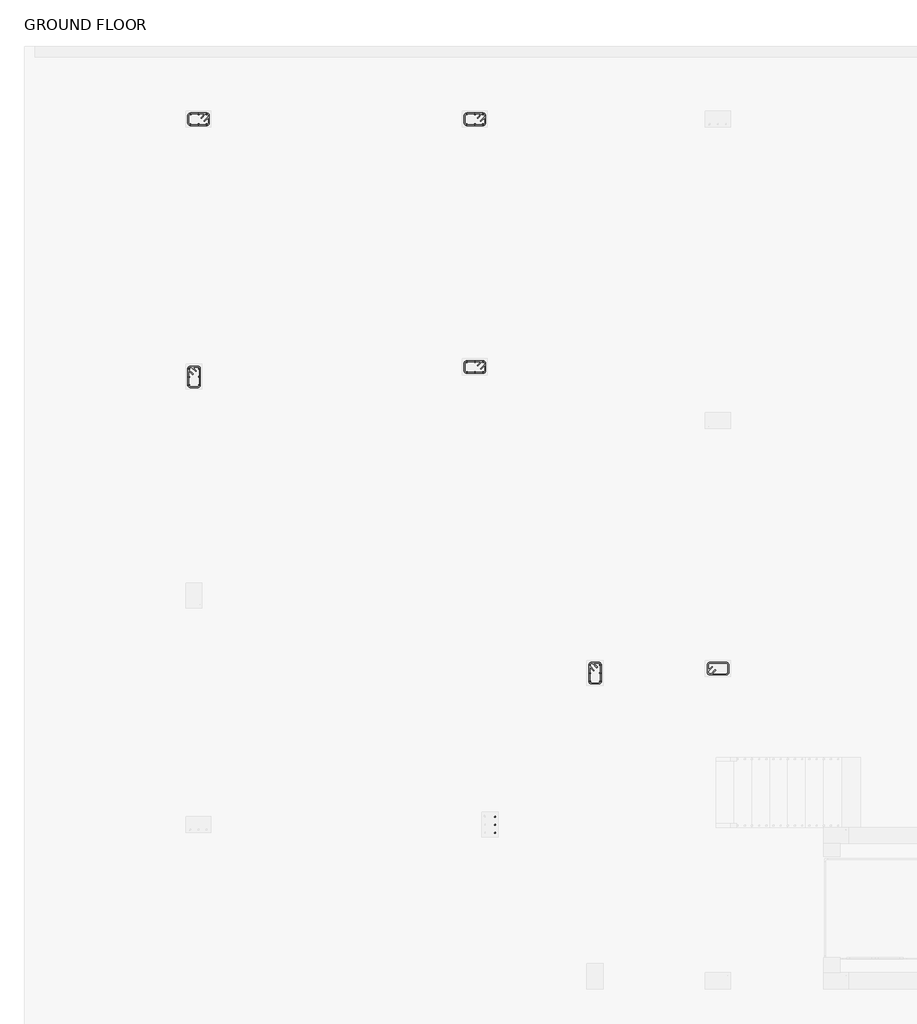
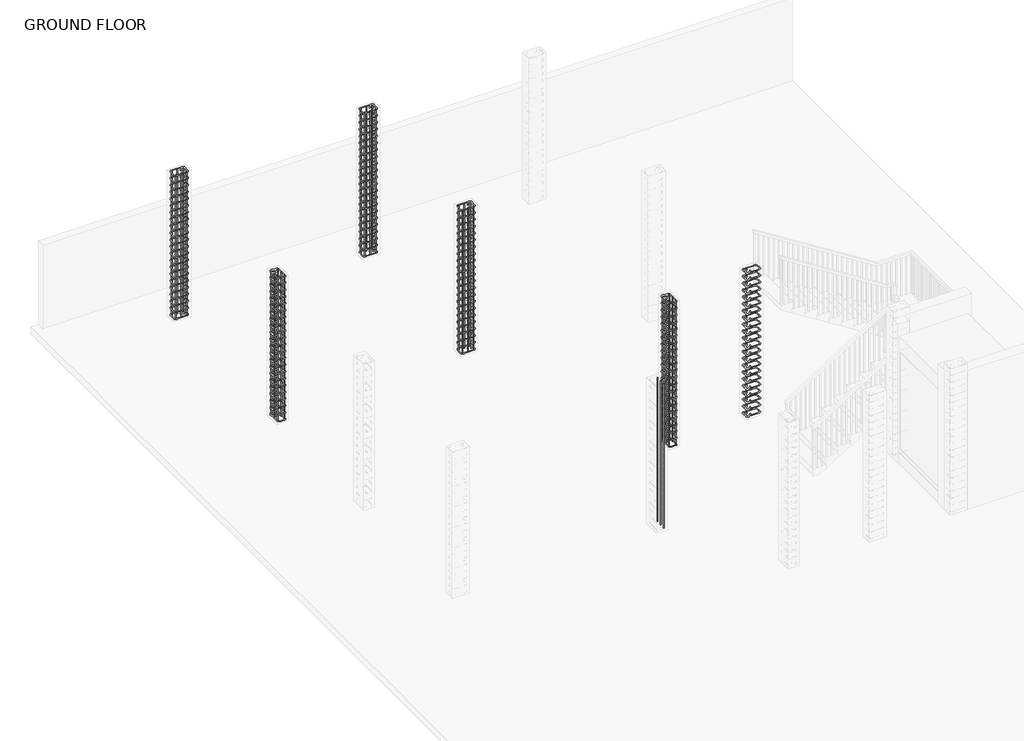
# One storey, part 6 of 7: 17 reinforcing bars.
"""IFC4 building model written with IfcOpenShell, lengths in millimetres."""

from ifc_helpers import new_model, si_unit, point, frame, origin, place, context, project, spatial, polyline, circle_curve, trimmed, segment, composite_curve, source, transform, mapped, element, save
from ifc_brep_helpers import swept_disk

model = new_model("IFC4")

# Units and contexts
model_context = context("Model", 3, world=origin())
ifc_project = project(units=[si_unit("LENGTHUNIT", "METRE", prefix="MILLI")], contexts=[model_context])

# Site, building, storey
site = spatial("IfcSite", under=ifc_project)
building = spatial("IfcBuilding", under=site)
storey = spatial("IfcBuildingStorey", under=building, Name="GROUND FLOOR", Elevation=0.0)

# Reinforcing bars
placement = place(None, origin())
reinforcing_bar_shape = source(origin(), model_context, "Body", "SolidModel", [
    swept_disk(composite_curve([segment(polyline([(-6036.4155558, 10049.1290376, 3168.65), (-5982.534019, 10103.0105743, 3168.65)]), True, "CONTINUOUS"), segment(trimmed(circle_curve(frame((-5960.0833787, 10080.559934, 3168.65), z_axis=(0.0, 0.0, -1.0), x_axis=(-22.450640299999577, 22.450640299999577, 0.0)), 31.75), [point((-5982.534019, 10103.0105743, 3168.65))], [point((-5928.3333787, 10080.559934, 3168.65))], True, "CARTESIAN"), True, "CONTINUOUS"), segment(polyline([(-5928.3333787, 10080.559934, 3168.65), (-5928.3333787, 9978.959934, 3168.65)]), True, "CONTINUOUS"), segment(trimmed(circle_curve(frame((-5960.0833787, 9978.959934, 3168.65), z_axis=(0.0, 0.0, -1.0), x_axis=(31.75, 0.0, 0.0)), 31.75), [point((-5928.3333787, 9978.959934, 3168.65))], [point((-5960.0833787, 9947.209934, 3168.65))], True, "CARTESIAN"), True, "CONTINUOUS"), segment(polyline([(-5960.0833787, 9947.209934, 3168.65), (-6188.6833787, 9947.209934, 3168.65)]), True, "CONTINUOUS"), segment(trimmed(circle_curve(frame((-6188.6833787, 9978.8664139, 3171.0851138), z_axis=(0.0, 0.07669649888473773, -0.9970544855015816), x_axis=(0.0, -31.656479899998885, -2.4351137999997263)), 31.75), [point((-6188.6833787, 9947.209934, 3168.65))], [point((-6220.4333787, 9978.8664139, 3171.0851138))], True, "CARTESIAN"), True, "CONTINUOUS"), segment(polyline([(-6220.4333787, 9978.8664139, 3171.0851138), (-6220.4333787, 10080.6534541, 3178.9148862)]), True, "CONTINUOUS"), segment(trimmed(circle_curve(frame((-6188.6833787, 10080.6534541, 3178.9148862), z_axis=(0.0, 0.07669649888473773, -0.9970544855015816), x_axis=(-31.75, 0.0, 0.0)), 31.75), [point((-6220.4333787, 10080.6534541, 3178.9148862))], [point((-6188.6833787, 10112.309934, 3181.35))], True, "CARTESIAN"), True, "CONTINUOUS"), segment(polyline([(-6188.6833787, 10112.309934, 3181.35), (-5960.0833787, 10112.309934, 3181.35)]), True, "CONTINUOUS"), segment(trimmed(circle_curve(frame((-5960.0833787, 10080.559934, 3181.35), z_axis=(0.0, 0.0, -1.0), x_axis=(0.0, 31.75, 0.0)), 31.75), [point((-5960.0833787, 10112.309934, 3181.35))], [point((-5937.6327384, 10058.1092937, 3181.35))], True, "CARTESIAN"), True, "CONTINUOUS"), segment(polyline([(-5937.6327384, 10058.1092937, 3181.35), (-5991.5142752, 10004.227757, 3181.35)]), True, "CONTINUOUS")], self_intersect=False), 6.35),
])
element("IfcReinforcingBar", 1, at=placement, inside=storey, context=model_context, shape_type="MappedRepresentation", body=[
    mapped(reinforcing_bar_shape, transform((0.0, 0.0, 0.0), x_axis=(1.0, 0.0, 0.0), y_axis=(0.0, 1.0, 0.0), z_axis=(0.0, 0.0, 1.0))),
    mapped(reinforcing_bar_shape, transform((0.0, 0.0, -149.3761905), x_axis=(1.0, 0.0, 0.0), y_axis=(0.0, 1.0, 0.0), z_axis=(0.0, 0.0, 1.0))),
    mapped(reinforcing_bar_shape, transform((0.0, 0.0, -298.752381), x_axis=(1.0, 0.0, 0.0), y_axis=(0.0, 1.0, 0.0), z_axis=(0.0, 0.0, 1.0))),
    mapped(reinforcing_bar_shape, transform((0.0, 0.0, -448.1285714), x_axis=(1.0, 0.0, 0.0), y_axis=(0.0, 1.0, 0.0), z_axis=(0.0, 0.0, 1.0))),
    mapped(reinforcing_bar_shape, transform((0.0, 0.0, -597.5047619), x_axis=(1.0, 0.0, 0.0), y_axis=(0.0, 1.0, 0.0), z_axis=(0.0, 0.0, 1.0))),
    mapped(reinforcing_bar_shape, transform((0.0, 0.0, -746.8809524), x_axis=(1.0, 0.0, 0.0), y_axis=(0.0, 1.0, 0.0), z_axis=(0.0, 0.0, 1.0))),
    mapped(reinforcing_bar_shape, transform((0.0, 0.0, -896.2571429), x_axis=(1.0, 0.0, 0.0), y_axis=(0.0, 1.0, 0.0), z_axis=(0.0, 0.0, 1.0))),
    mapped(reinforcing_bar_shape, transform((0.0, 0.0, -1045.6333333), x_axis=(1.0, 0.0, 0.0), y_axis=(0.0, 1.0, 0.0), z_axis=(0.0, 0.0, 1.0))),
    mapped(reinforcing_bar_shape, transform((0.0, 0.0, -1195.0095238), x_axis=(1.0, 0.0, 0.0), y_axis=(0.0, 1.0, 0.0), z_axis=(0.0, 0.0, 1.0))),
    mapped(reinforcing_bar_shape, transform((0.0, 0.0, -1344.3857143), x_axis=(1.0, 0.0, 0.0), y_axis=(0.0, 1.0, 0.0), z_axis=(0.0, 0.0, 1.0))),
    mapped(reinforcing_bar_shape, transform((0.0, 0.0, -1493.7619048), x_axis=(1.0, 0.0, 0.0), y_axis=(0.0, 1.0, 0.0), z_axis=(0.0, 0.0, 1.0))),
    mapped(reinforcing_bar_shape, transform((0.0, 0.0, -1643.1380952), x_axis=(1.0, 0.0, 0.0), y_axis=(0.0, 1.0, 0.0), z_axis=(0.0, 0.0, 1.0))),
    mapped(reinforcing_bar_shape, transform((0.0, 0.0, -1792.5142857), x_axis=(1.0, 0.0, 0.0), y_axis=(0.0, 1.0, 0.0), z_axis=(0.0, 0.0, 1.0))),
    mapped(reinforcing_bar_shape, transform((0.0, 0.0, -1941.8904762), x_axis=(1.0, 0.0, 0.0), y_axis=(0.0, 1.0, 0.0), z_axis=(0.0, 0.0, 1.0))),
    mapped(reinforcing_bar_shape, transform((0.0, 0.0, -2091.2666667), x_axis=(1.0, 0.0, 0.0), y_axis=(0.0, 1.0, 0.0), z_axis=(0.0, 0.0, 1.0))),
    mapped(reinforcing_bar_shape, transform((0.0, 0.0, -2240.6428571), x_axis=(1.0, 0.0, 0.0), y_axis=(0.0, 1.0, 0.0), z_axis=(0.0, 0.0, 1.0))),
    mapped(reinforcing_bar_shape, transform((0.0, 0.0, -2390.0190476), x_axis=(1.0, 0.0, 0.0), y_axis=(0.0, 1.0, 0.0), z_axis=(0.0, 0.0, 1.0))),
    mapped(reinforcing_bar_shape, transform((0.0, 0.0, -2539.3952381), x_axis=(1.0, 0.0, 0.0), y_axis=(0.0, 1.0, 0.0), z_axis=(0.0, 0.0, 1.0))),
    mapped(reinforcing_bar_shape, transform((0.0, 0.0, -2688.7714286), x_axis=(1.0, 0.0, 0.0), y_axis=(0.0, 1.0, 0.0), z_axis=(0.0, 0.0, 1.0))),
    mapped(reinforcing_bar_shape, transform((0.0, 0.0, -2838.147619), x_axis=(1.0, 0.0, 0.0), y_axis=(0.0, 1.0, 0.0), z_axis=(0.0, 0.0, 1.0))),
    mapped(reinforcing_bar_shape, transform((0.0, 0.0, -2987.5238095), x_axis=(1.0, 0.0, 0.0), y_axis=(0.0, 1.0, 0.0), z_axis=(0.0, 0.0, 1.0))),
    mapped(reinforcing_bar_shape, transform((0.0, 0.0, -3136.9), x_axis=(1.0, 0.0, 0.0), y_axis=(0.0, 1.0, 0.0), z_axis=(0.0, 0.0, 1.0))),
])
reinforcing_bar_2_shape = source(origin(), model_context, "Body", "SolidModel", [
    swept_disk(composite_curve([segment(polyline([(-5960.0833787, 9959.909934, 3175.0), (-5960.0833787, 9959.909934, 25.4)]), True, "CONTINUOUS")], self_intersect=False), 6.35),
])
element("IfcReinforcingBar", 2, at=placement, inside=storey, context=model_context, shape_type="MappedRepresentation", body=[
    mapped(reinforcing_bar_2_shape, transform((0.0, 0.0, 0.0), x_axis=(1.0, 0.0, 0.0), y_axis=(0.0, 1.0, 0.0), z_axis=(0.0, 0.0, 1.0))),
    mapped(reinforcing_bar_2_shape, transform((-114.3, 0.0, 0.0), x_axis=(1.0, 0.0, 0.0), y_axis=(0.0, 1.0, 0.0), z_axis=(0.0, 0.0, 1.0))),
    mapped(reinforcing_bar_2_shape, transform((-228.6, 0.0, 0.0), x_axis=(1.0, 0.0, 0.0), y_axis=(0.0, 1.0, 0.0), z_axis=(0.0, 0.0, 1.0))),
])
reinforcing_bar_3_shape = source(origin(), model_context, "Body", "SolidModel", [
    swept_disk(composite_curve([segment(polyline([(-5960.0833787, 10099.609934, 25.4), (-5960.0833787, 10099.609934, 3175.0)]), True, "CONTINUOUS")], self_intersect=False), 6.35),
])
element("IfcReinforcingBar", 3, at=placement, inside=storey, context=model_context, shape_type="MappedRepresentation", body=[
    mapped(reinforcing_bar_3_shape, transform((0.0, 0.0, 0.0), x_axis=(1.0, 0.0, 0.0), y_axis=(0.0, 1.0, 0.0), z_axis=(0.0, 0.0, 1.0))),
    mapped(reinforcing_bar_3_shape, transform((-114.3, 0.0, 0.0), x_axis=(1.0, 0.0, 0.0), y_axis=(0.0, 1.0, 0.0), z_axis=(0.0, 0.0, 1.0))),
    mapped(reinforcing_bar_3_shape, transform((-228.6, 0.0, 0.0), x_axis=(1.0, 0.0, 0.0), y_axis=(0.0, 1.0, 0.0), z_axis=(0.0, 0.0, 1.0))),
])
reinforcing_bar_4_shape = source(origin(), model_context, "Body", "SolidModel", [
    swept_disk(composite_curve([segment(polyline([(-2124.8155558, 10049.1290376, 3168.65), (-2070.934019, 10103.0105743, 3168.65)]), True, "CONTINUOUS"), segment(trimmed(circle_curve(frame((-2048.4833787, 10080.559934, 3168.65), z_axis=(0.0, 0.0, -1.0), x_axis=(-22.450640300000032, 22.450640299999577, 0.0)), 31.75), [point((-2070.934019, 10103.0105743, 3168.65))], [point((-2016.7333787, 10080.559934, 3168.65))], True, "CARTESIAN"), True, "CONTINUOUS"), segment(polyline([(-2016.7333787, 10080.559934, 3168.65), (-2016.7333787, 9978.959934, 3168.65)]), True, "CONTINUOUS"), segment(trimmed(circle_curve(frame((-2048.4833787, 9978.959934, 3168.65), z_axis=(0.0, 0.0, -1.0), x_axis=(31.749999999999773, 0.0, 0.0)), 31.75), [point((-2016.7333787, 9978.959934, 3168.65))], [point((-2048.4833787, 9947.209934, 3168.65))], True, "CARTESIAN"), True, "CONTINUOUS"), segment(polyline([(-2048.4833787, 9947.209934, 3168.65), (-2277.0833787, 9947.209934, 3168.65)]), True, "CONTINUOUS"), segment(trimmed(circle_curve(frame((-2277.0833787, 9978.8664139, 3171.0851138), z_axis=(0.0, 0.07669649888473773, -0.9970544855015816), x_axis=(0.0, -31.656479899998885, -2.4351137999997263)), 31.75), [point((-2277.0833787, 9947.209934, 3168.65))], [point((-2308.8333787, 9978.8664139, 3171.0851138))], True, "CARTESIAN"), True, "CONTINUOUS"), segment(polyline([(-2308.8333787, 9978.8664139, 3171.0851138), (-2308.8333787, 10080.6534541, 3178.9148862)]), True, "CONTINUOUS"), segment(trimmed(circle_curve(frame((-2277.0833787, 10080.6534541, 3178.9148862), z_axis=(0.0, 0.07669649888473773, -0.9970544855015816), x_axis=(-31.75, 0.0, 0.0)), 31.75), [point((-2308.8333787, 10080.6534541, 3178.9148862))], [point((-2277.0833787, 10112.309934, 3181.35))], True, "CARTESIAN"), True, "CONTINUOUS"), segment(polyline([(-2277.0833787, 10112.309934, 3181.35), (-2048.4833787, 10112.309934, 3181.35)]), True, "CONTINUOUS"), segment(trimmed(circle_curve(frame((-2048.4833787, 10080.559934, 3181.35), z_axis=(0.0, 0.0, -1.0), x_axis=(0.0, 31.75, 0.0)), 31.75), [point((-2048.4833787, 10112.309934, 3181.35))], [point((-2026.0327384, 10058.1092937, 3181.35))], True, "CARTESIAN"), True, "CONTINUOUS"), segment(polyline([(-2026.0327384, 10058.1092937, 3181.35), (-2079.9142752, 10004.227757, 3181.35)]), True, "CONTINUOUS")], self_intersect=False), 6.35),
])
element("IfcReinforcingBar", 4, at=placement, inside=storey, context=model_context, shape_type="MappedRepresentation", body=[
    mapped(reinforcing_bar_4_shape, transform((0.0, 0.0, 0.0), x_axis=(1.0, 0.0, 0.0), y_axis=(0.0, 1.0, 0.0), z_axis=(0.0, 0.0, 1.0))),
    mapped(reinforcing_bar_4_shape, transform((0.0, 0.0, -149.3761905), x_axis=(1.0, 0.0, 0.0), y_axis=(0.0, 1.0, 0.0), z_axis=(0.0, 0.0, 1.0))),
    mapped(reinforcing_bar_4_shape, transform((0.0, 0.0, -298.752381), x_axis=(1.0, 0.0, 0.0), y_axis=(0.0, 1.0, 0.0), z_axis=(0.0, 0.0, 1.0))),
    mapped(reinforcing_bar_4_shape, transform((0.0, 0.0, -448.1285714), x_axis=(1.0, 0.0, 0.0), y_axis=(0.0, 1.0, 0.0), z_axis=(0.0, 0.0, 1.0))),
    mapped(reinforcing_bar_4_shape, transform((0.0, 0.0, -597.5047619), x_axis=(1.0, 0.0, 0.0), y_axis=(0.0, 1.0, 0.0), z_axis=(0.0, 0.0, 1.0))),
    mapped(reinforcing_bar_4_shape, transform((0.0, 0.0, -746.8809524), x_axis=(1.0, 0.0, 0.0), y_axis=(0.0, 1.0, 0.0), z_axis=(0.0, 0.0, 1.0))),
    mapped(reinforcing_bar_4_shape, transform((0.0, 0.0, -896.2571429), x_axis=(1.0, 0.0, 0.0), y_axis=(0.0, 1.0, 0.0), z_axis=(0.0, 0.0, 1.0))),
    mapped(reinforcing_bar_4_shape, transform((0.0, 0.0, -1045.6333333), x_axis=(1.0, 0.0, 0.0), y_axis=(0.0, 1.0, 0.0), z_axis=(0.0, 0.0, 1.0))),
    mapped(reinforcing_bar_4_shape, transform((0.0, 0.0, -1195.0095238), x_axis=(1.0, 0.0, 0.0), y_axis=(0.0, 1.0, 0.0), z_axis=(0.0, 0.0, 1.0))),
    mapped(reinforcing_bar_4_shape, transform((0.0, 0.0, -1344.3857143), x_axis=(1.0, 0.0, 0.0), y_axis=(0.0, 1.0, 0.0), z_axis=(0.0, 0.0, 1.0))),
    mapped(reinforcing_bar_4_shape, transform((0.0, 0.0, -1493.7619048), x_axis=(1.0, 0.0, 0.0), y_axis=(0.0, 1.0, 0.0), z_axis=(0.0, 0.0, 1.0))),
    mapped(reinforcing_bar_4_shape, transform((0.0, 0.0, -1643.1380952), x_axis=(1.0, 0.0, 0.0), y_axis=(0.0, 1.0, 0.0), z_axis=(0.0, 0.0, 1.0))),
    mapped(reinforcing_bar_4_shape, transform((0.0, 0.0, -1792.5142857), x_axis=(1.0, 0.0, 0.0), y_axis=(0.0, 1.0, 0.0), z_axis=(0.0, 0.0, 1.0))),
    mapped(reinforcing_bar_4_shape, transform((0.0, 0.0, -1941.8904762), x_axis=(1.0, 0.0, 0.0), y_axis=(0.0, 1.0, 0.0), z_axis=(0.0, 0.0, 1.0))),
    mapped(reinforcing_bar_4_shape, transform((0.0, 0.0, -2091.2666667), x_axis=(1.0, 0.0, 0.0), y_axis=(0.0, 1.0, 0.0), z_axis=(0.0, 0.0, 1.0))),
    mapped(reinforcing_bar_4_shape, transform((0.0, 0.0, -2240.6428571), x_axis=(1.0, 0.0, 0.0), y_axis=(0.0, 1.0, 0.0), z_axis=(0.0, 0.0, 1.0))),
    mapped(reinforcing_bar_4_shape, transform((0.0, 0.0, -2390.0190476), x_axis=(1.0, 0.0, 0.0), y_axis=(0.0, 1.0, 0.0), z_axis=(0.0, 0.0, 1.0))),
    mapped(reinforcing_bar_4_shape, transform((0.0, 0.0, -2539.3952381), x_axis=(1.0, 0.0, 0.0), y_axis=(0.0, 1.0, 0.0), z_axis=(0.0, 0.0, 1.0))),
    mapped(reinforcing_bar_4_shape, transform((0.0, 0.0, -2688.7714286), x_axis=(1.0, 0.0, 0.0), y_axis=(0.0, 1.0, 0.0), z_axis=(0.0, 0.0, 1.0))),
    mapped(reinforcing_bar_4_shape, transform((0.0, 0.0, -2838.147619), x_axis=(1.0, 0.0, 0.0), y_axis=(0.0, 1.0, 0.0), z_axis=(0.0, 0.0, 1.0))),
    mapped(reinforcing_bar_4_shape, transform((0.0, 0.0, -2987.5238095), x_axis=(1.0, 0.0, 0.0), y_axis=(0.0, 1.0, 0.0), z_axis=(0.0, 0.0, 1.0))),
    mapped(reinforcing_bar_4_shape, transform((0.0, 0.0, -3136.9), x_axis=(1.0, 0.0, 0.0), y_axis=(0.0, 1.0, 0.0), z_axis=(0.0, 0.0, 1.0))),
])
reinforcing_bar_5_shape = source(origin(), model_context, "Body", "SolidModel", [
    swept_disk(composite_curve([segment(polyline([(-2048.4833787, 9959.909934, 3175.0), (-2048.4833787, 9959.909934, 25.4)]), True, "CONTINUOUS")], self_intersect=False), 6.35),
])
element("IfcReinforcingBar", 5, at=placement, inside=storey, context=model_context, shape_type="MappedRepresentation", body=[
    mapped(reinforcing_bar_5_shape, transform((0.0, 0.0, 0.0), x_axis=(1.0, 0.0, 0.0), y_axis=(0.0, 1.0, 0.0), z_axis=(0.0, 0.0, 1.0))),
    mapped(reinforcing_bar_5_shape, transform((-114.3, 0.0, 0.0), x_axis=(1.0, 0.0, 0.0), y_axis=(0.0, 1.0, 0.0), z_axis=(0.0, 0.0, 1.0))),
    mapped(reinforcing_bar_5_shape, transform((-228.6, 0.0, 0.0), x_axis=(1.0, 0.0, 0.0), y_axis=(0.0, 1.0, 0.0), z_axis=(0.0, 0.0, 1.0))),
])
reinforcing_bar_6_shape = source(origin(), model_context, "Body", "SolidModel", [
    swept_disk(composite_curve([segment(polyline([(-2048.4833787, 10099.609934, 25.4), (-2048.4833787, 10099.609934, 3175.0)]), True, "CONTINUOUS")], self_intersect=False), 6.35),
])
element("IfcReinforcingBar", 6, at=placement, inside=storey, context=model_context, shape_type="MappedRepresentation", body=[
    mapped(reinforcing_bar_6_shape, transform((0.0, 0.0, 0.0), x_axis=(1.0, 0.0, 0.0), y_axis=(0.0, 1.0, 0.0), z_axis=(0.0, 0.0, 1.0))),
    mapped(reinforcing_bar_6_shape, transform((-114.3, 0.0, 0.0), x_axis=(1.0, 0.0, 0.0), y_axis=(0.0, 1.0, 0.0), z_axis=(0.0, 0.0, 1.0))),
    mapped(reinforcing_bar_6_shape, transform((-228.6, 0.0, 0.0), x_axis=(1.0, 0.0, 0.0), y_axis=(0.0, 1.0, 0.0), z_axis=(0.0, 0.0, 1.0))),
])
reinforcing_bar_7_shape = source(origin(), model_context, "Body", "SolidModel", [
    swept_disk(composite_curve([segment(polyline([(-2124.8155558, 6543.9290376, 3168.65), (-2070.934019, 6597.8105743, 3168.65)]), True, "CONTINUOUS"), segment(trimmed(circle_curve(frame((-2048.4833787, 6575.359934, 3168.65), z_axis=(0.0, 0.0, -1.0), x_axis=(-22.450640300000032, 22.450640299999577, 0.0)), 31.75), [point((-2070.934019, 6597.8105743, 3168.65))], [point((-2016.7333787, 6575.359934, 3168.65))], True, "CARTESIAN"), True, "CONTINUOUS"), segment(polyline([(-2016.7333787, 6575.359934, 3168.65), (-2016.7333787, 6473.759934, 3168.65)]), True, "CONTINUOUS"), segment(trimmed(circle_curve(frame((-2048.4833787, 6473.759934, 3168.65), z_axis=(0.0, 0.0, -1.0), x_axis=(31.749999999999773, 0.0, 0.0)), 31.75), [point((-2016.7333787, 6473.759934, 3168.65))], [point((-2048.4833787, 6442.009934, 3168.65))], True, "CARTESIAN"), True, "CONTINUOUS"), segment(polyline([(-2048.4833787, 6442.009934, 3168.65), (-2277.0833787, 6442.009934, 3168.65)]), True, "CONTINUOUS"), segment(trimmed(circle_curve(frame((-2277.0833787, 6473.6664139, 3171.0851138), z_axis=(0.0, 0.07669649888473773, -0.9970544855015816), x_axis=(0.0, -31.656479900000704, -2.4351137999997263)), 31.75), [point((-2277.0833787, 6442.009934, 3168.65))], [point((-2308.8333787, 6473.6664139, 3171.0851138))], True, "CARTESIAN"), True, "CONTINUOUS"), segment(polyline([(-2308.8333787, 6473.6664139, 3171.0851138), (-2308.8333787, 6575.4534541, 3178.9148862)]), True, "CONTINUOUS"), segment(trimmed(circle_curve(frame((-2277.0833787, 6575.4534541, 3178.9148862), z_axis=(0.0, 0.07669649888473773, -0.9970544855015816), x_axis=(-31.75, 0.0, 0.0)), 31.75), [point((-2308.8333787, 6575.4534541, 3178.9148862))], [point((-2277.0833787, 6607.109934, 3181.35))], True, "CARTESIAN"), True, "CONTINUOUS"), segment(polyline([(-2277.0833787, 6607.109934, 3181.35), (-2048.4833787, 6607.109934, 3181.35)]), True, "CONTINUOUS"), segment(trimmed(circle_curve(frame((-2048.4833787, 6575.359934, 3181.35), z_axis=(0.0, 0.0, -1.0), x_axis=(0.0, 31.75, 0.0)), 31.75), [point((-2048.4833787, 6607.109934, 3181.35))], [point((-2026.0327384, 6552.9092937, 3181.35))], True, "CARTESIAN"), True, "CONTINUOUS"), segment(polyline([(-2026.0327384, 6552.9092937, 3181.35), (-2079.9142752, 6499.027757, 3181.35)]), True, "CONTINUOUS")], self_intersect=False), 6.35),
])
element("IfcReinforcingBar", 7, at=placement, inside=storey, context=model_context, shape_type="MappedRepresentation", body=[
    mapped(reinforcing_bar_7_shape, transform((0.0, 0.0, 0.0), x_axis=(1.0, 0.0, 0.0), y_axis=(0.0, 1.0, 0.0), z_axis=(0.0, 0.0, 1.0))),
    mapped(reinforcing_bar_7_shape, transform((0.0, 0.0, -149.3761905), x_axis=(1.0, 0.0, 0.0), y_axis=(0.0, 1.0, 0.0), z_axis=(0.0, 0.0, 1.0))),
    mapped(reinforcing_bar_7_shape, transform((0.0, 0.0, -298.752381), x_axis=(1.0, 0.0, 0.0), y_axis=(0.0, 1.0, 0.0), z_axis=(0.0, 0.0, 1.0))),
    mapped(reinforcing_bar_7_shape, transform((0.0, 0.0, -448.1285714), x_axis=(1.0, 0.0, 0.0), y_axis=(0.0, 1.0, 0.0), z_axis=(0.0, 0.0, 1.0))),
    mapped(reinforcing_bar_7_shape, transform((0.0, 0.0, -597.5047619), x_axis=(1.0, 0.0, 0.0), y_axis=(0.0, 1.0, 0.0), z_axis=(0.0, 0.0, 1.0))),
    mapped(reinforcing_bar_7_shape, transform((0.0, 0.0, -746.8809524), x_axis=(1.0, 0.0, 0.0), y_axis=(0.0, 1.0, 0.0), z_axis=(0.0, 0.0, 1.0))),
    mapped(reinforcing_bar_7_shape, transform((0.0, 0.0, -896.2571429), x_axis=(1.0, 0.0, 0.0), y_axis=(0.0, 1.0, 0.0), z_axis=(0.0, 0.0, 1.0))),
    mapped(reinforcing_bar_7_shape, transform((0.0, 0.0, -1045.6333333), x_axis=(1.0, 0.0, 0.0), y_axis=(0.0, 1.0, 0.0), z_axis=(0.0, 0.0, 1.0))),
    mapped(reinforcing_bar_7_shape, transform((0.0, 0.0, -1195.0095238), x_axis=(1.0, 0.0, 0.0), y_axis=(0.0, 1.0, 0.0), z_axis=(0.0, 0.0, 1.0))),
    mapped(reinforcing_bar_7_shape, transform((0.0, 0.0, -1344.3857143), x_axis=(1.0, 0.0, 0.0), y_axis=(0.0, 1.0, 0.0), z_axis=(0.0, 0.0, 1.0))),
    mapped(reinforcing_bar_7_shape, transform((0.0, 0.0, -1493.7619048), x_axis=(1.0, 0.0, 0.0), y_axis=(0.0, 1.0, 0.0), z_axis=(0.0, 0.0, 1.0))),
    mapped(reinforcing_bar_7_shape, transform((0.0, 0.0, -1643.1380952), x_axis=(1.0, 0.0, 0.0), y_axis=(0.0, 1.0, 0.0), z_axis=(0.0, 0.0, 1.0))),
    mapped(reinforcing_bar_7_shape, transform((0.0, 0.0, -1792.5142857), x_axis=(1.0, 0.0, 0.0), y_axis=(0.0, 1.0, 0.0), z_axis=(0.0, 0.0, 1.0))),
    mapped(reinforcing_bar_7_shape, transform((0.0, 0.0, -1941.8904762), x_axis=(1.0, 0.0, 0.0), y_axis=(0.0, 1.0, 0.0), z_axis=(0.0, 0.0, 1.0))),
    mapped(reinforcing_bar_7_shape, transform((0.0, 0.0, -2091.2666667), x_axis=(1.0, 0.0, 0.0), y_axis=(0.0, 1.0, 0.0), z_axis=(0.0, 0.0, 1.0))),
    mapped(reinforcing_bar_7_shape, transform((0.0, 0.0, -2240.6428571), x_axis=(1.0, 0.0, 0.0), y_axis=(0.0, 1.0, 0.0), z_axis=(0.0, 0.0, 1.0))),
    mapped(reinforcing_bar_7_shape, transform((0.0, 0.0, -2390.0190476), x_axis=(1.0, 0.0, 0.0), y_axis=(0.0, 1.0, 0.0), z_axis=(0.0, 0.0, 1.0))),
    mapped(reinforcing_bar_7_shape, transform((0.0, 0.0, -2539.3952381), x_axis=(1.0, 0.0, 0.0), y_axis=(0.0, 1.0, 0.0), z_axis=(0.0, 0.0, 1.0))),
    mapped(reinforcing_bar_7_shape, transform((0.0, 0.0, -2688.7714286), x_axis=(1.0, 0.0, 0.0), y_axis=(0.0, 1.0, 0.0), z_axis=(0.0, 0.0, 1.0))),
    mapped(reinforcing_bar_7_shape, transform((0.0, 0.0, -2838.147619), x_axis=(1.0, 0.0, 0.0), y_axis=(0.0, 1.0, 0.0), z_axis=(0.0, 0.0, 1.0))),
    mapped(reinforcing_bar_7_shape, transform((0.0, 0.0, -2987.5238095), x_axis=(1.0, 0.0, 0.0), y_axis=(0.0, 1.0, 0.0), z_axis=(0.0, 0.0, 1.0))),
    mapped(reinforcing_bar_7_shape, transform((0.0, 0.0, -3136.9), x_axis=(1.0, 0.0, 0.0), y_axis=(0.0, 1.0, 0.0), z_axis=(0.0, 0.0, 1.0))),
])
reinforcing_bar_8_shape = source(origin(), model_context, "Body", "SolidModel", [
    swept_disk(composite_curve([segment(polyline([(-2048.4833787, 6454.709934, 3175.0), (-2048.4833787, 6454.709934, 25.4)]), True, "CONTINUOUS")], self_intersect=False), 6.35),
])
element("IfcReinforcingBar", 8, at=placement, inside=storey, context=model_context, shape_type="MappedRepresentation", body=[
    mapped(reinforcing_bar_8_shape, transform((0.0, 0.0, 0.0), x_axis=(1.0, 0.0, 0.0), y_axis=(0.0, 1.0, 0.0), z_axis=(0.0, 0.0, 1.0))),
    mapped(reinforcing_bar_8_shape, transform((-114.3, 0.0, 0.0), x_axis=(1.0, 0.0, 0.0), y_axis=(0.0, 1.0, 0.0), z_axis=(0.0, 0.0, 1.0))),
    mapped(reinforcing_bar_8_shape, transform((-228.6, 0.0, 0.0), x_axis=(1.0, 0.0, 0.0), y_axis=(0.0, 1.0, 0.0), z_axis=(0.0, 0.0, 1.0))),
])
reinforcing_bar_9_shape = source(origin(), model_context, "Body", "SolidModel", [
    swept_disk(composite_curve([segment(polyline([(-2048.4833787, 6594.409934, 25.4), (-2048.4833787, 6594.409934, 3175.0)]), True, "CONTINUOUS")], self_intersect=False), 6.35),
])
element("IfcReinforcingBar", 9, at=placement, inside=storey, context=model_context, shape_type="MappedRepresentation", body=[
    mapped(reinforcing_bar_9_shape, transform((0.0, 0.0, 0.0), x_axis=(1.0, 0.0, 0.0), y_axis=(0.0, 1.0, 0.0), z_axis=(0.0, 0.0, 1.0))),
    mapped(reinforcing_bar_9_shape, transform((-114.3, 0.0, 0.0), x_axis=(1.0, 0.0, 0.0), y_axis=(0.0, 1.0, 0.0), z_axis=(0.0, 0.0, 1.0))),
    mapped(reinforcing_bar_9_shape, transform((-228.6, 0.0, 0.0), x_axis=(1.0, 0.0, 0.0), y_axis=(0.0, 1.0, 0.0), z_axis=(0.0, 0.0, 1.0))),
])
reinforcing_bar_10_shape = source(origin(), model_context, "Body", "SolidModel", [
    swept_disk(composite_curve([segment(polyline([(-6157.2524823, 6422.827757, 3168.65), (-6211.134019, 6476.7092937, 3168.65)]), True, "CONTINUOUS"), segment(trimmed(circle_curve(frame((-6188.6833787, 6499.159934, 3168.65), z_axis=(0.0, 0.0, -1.0), x_axis=(-22.450640300000487, -22.450640300000487, 0.0)), 31.75), [point((-6211.134019, 6476.7092937, 3168.65))], [point((-6188.6833787, 6530.909934, 3168.65))], True, "CARTESIAN"), True, "CONTINUOUS"), segment(polyline([(-6188.6833787, 6530.909934, 3168.65), (-6087.0833787, 6530.909934, 3168.65)]), True, "CONTINUOUS"), segment(trimmed(circle_curve(frame((-6087.0833787, 6499.159934, 3168.65), z_axis=(0.0, 0.0, -1.0), x_axis=(0.0, 31.75, 0.0)), 31.75), [point((-6087.0833787, 6530.909934, 3168.65))], [point((-6055.3333787, 6499.159934, 3168.65))], True, "CARTESIAN"), True, "CONTINUOUS"), segment(polyline([(-6055.3333787, 6499.159934, 3168.65), (-6055.3333787, 6270.559934, 3168.65)]), True, "CONTINUOUS"), segment(trimmed(circle_curve(frame((-6086.9898586, 6270.559934, 3171.0851138), z_axis=(-0.07669649888473773, 0.0, -0.9970544855015816), x_axis=(31.656479899999795, 0.0, -2.4351137999997263)), 31.75), [point((-6055.3333787, 6270.559934, 3168.65))], [point((-6086.9898586, 6238.809934, 3171.0851138))], True, "CARTESIAN"), True, "CONTINUOUS"), segment(polyline([(-6086.9898586, 6238.809934, 3171.0851138), (-6188.7768988, 6238.809934, 3178.9148862)]), True, "CONTINUOUS"), segment(trimmed(circle_curve(frame((-6188.7768988, 6270.559934, 3178.9148862), z_axis=(-0.07669649888473773, 0.0, -0.9970544855015816), x_axis=(0.0, -31.75, 0.0)), 31.75), [point((-6188.7768988, 6238.809934, 3178.9148862))], [point((-6220.4333787, 6270.559934, 3181.35))], True, "CARTESIAN"), True, "CONTINUOUS"), segment(polyline([(-6220.4333787, 6270.559934, 3181.35), (-6220.4333787, 6499.159934, 3181.35)]), True, "CONTINUOUS"), segment(trimmed(circle_curve(frame((-6188.6833787, 6499.159934, 3181.35), z_axis=(0.0, 0.0, -1.0), x_axis=(-31.75, 0.0, 0.0)), 31.75), [point((-6220.4333787, 6499.159934, 3181.35))], [point((-6166.2327384, 6521.6105743, 3181.35))], True, "CARTESIAN"), True, "CONTINUOUS"), segment(polyline([(-6166.2327384, 6521.6105743, 3181.35), (-6112.3512017, 6467.7290376, 3181.35)]), True, "CONTINUOUS")], self_intersect=False), 6.35),
])
element("IfcReinforcingBar", 10, at=placement, inside=storey, context=model_context, shape_type="MappedRepresentation", body=[
    mapped(reinforcing_bar_10_shape, transform((0.0, 0.0, 0.0), x_axis=(1.0, 0.0, 0.0), y_axis=(0.0, 1.0, 0.0), z_axis=(0.0, 0.0, 1.0))),
    mapped(reinforcing_bar_10_shape, transform((0.0, 0.0, -149.3761905), x_axis=(1.0, 0.0, 0.0), y_axis=(0.0, 1.0, 0.0), z_axis=(0.0, 0.0, 1.0))),
    mapped(reinforcing_bar_10_shape, transform((0.0, 0.0, -298.752381), x_axis=(1.0, 0.0, 0.0), y_axis=(0.0, 1.0, 0.0), z_axis=(0.0, 0.0, 1.0))),
    mapped(reinforcing_bar_10_shape, transform((0.0, 0.0, -448.1285714), x_axis=(1.0, 0.0, 0.0), y_axis=(0.0, 1.0, 0.0), z_axis=(0.0, 0.0, 1.0))),
    mapped(reinforcing_bar_10_shape, transform((0.0, 0.0, -597.5047619), x_axis=(1.0, 0.0, 0.0), y_axis=(0.0, 1.0, 0.0), z_axis=(0.0, 0.0, 1.0))),
    mapped(reinforcing_bar_10_shape, transform((0.0, 0.0, -746.8809524), x_axis=(1.0, 0.0, 0.0), y_axis=(0.0, 1.0, 0.0), z_axis=(0.0, 0.0, 1.0))),
    mapped(reinforcing_bar_10_shape, transform((0.0, 0.0, -896.2571429), x_axis=(1.0, 0.0, 0.0), y_axis=(0.0, 1.0, 0.0), z_axis=(0.0, 0.0, 1.0))),
    mapped(reinforcing_bar_10_shape, transform((0.0, 0.0, -1045.6333333), x_axis=(1.0, 0.0, 0.0), y_axis=(0.0, 1.0, 0.0), z_axis=(0.0, 0.0, 1.0))),
    mapped(reinforcing_bar_10_shape, transform((0.0, 0.0, -1195.0095238), x_axis=(1.0, 0.0, 0.0), y_axis=(0.0, 1.0, 0.0), z_axis=(0.0, 0.0, 1.0))),
    mapped(reinforcing_bar_10_shape, transform((0.0, 0.0, -1344.3857143), x_axis=(1.0, 0.0, 0.0), y_axis=(0.0, 1.0, 0.0), z_axis=(0.0, 0.0, 1.0))),
    mapped(reinforcing_bar_10_shape, transform((0.0, 0.0, -1493.7619048), x_axis=(1.0, 0.0, 0.0), y_axis=(0.0, 1.0, 0.0), z_axis=(0.0, 0.0, 1.0))),
    mapped(reinforcing_bar_10_shape, transform((0.0, 0.0, -1643.1380952), x_axis=(1.0, 0.0, 0.0), y_axis=(0.0, 1.0, 0.0), z_axis=(0.0, 0.0, 1.0))),
    mapped(reinforcing_bar_10_shape, transform((0.0, 0.0, -1792.5142857), x_axis=(1.0, 0.0, 0.0), y_axis=(0.0, 1.0, 0.0), z_axis=(0.0, 0.0, 1.0))),
    mapped(reinforcing_bar_10_shape, transform((0.0, 0.0, -1941.8904762), x_axis=(1.0, 0.0, 0.0), y_axis=(0.0, 1.0, 0.0), z_axis=(0.0, 0.0, 1.0))),
    mapped(reinforcing_bar_10_shape, transform((0.0, 0.0, -2091.2666667), x_axis=(1.0, 0.0, 0.0), y_axis=(0.0, 1.0, 0.0), z_axis=(0.0, 0.0, 1.0))),
    mapped(reinforcing_bar_10_shape, transform((0.0, 0.0, -2240.6428571), x_axis=(1.0, 0.0, 0.0), y_axis=(0.0, 1.0, 0.0), z_axis=(0.0, 0.0, 1.0))),
    mapped(reinforcing_bar_10_shape, transform((0.0, 0.0, -2390.0190476), x_axis=(1.0, 0.0, 0.0), y_axis=(0.0, 1.0, 0.0), z_axis=(0.0, 0.0, 1.0))),
    mapped(reinforcing_bar_10_shape, transform((0.0, 0.0, -2539.3952381), x_axis=(1.0, 0.0, 0.0), y_axis=(0.0, 1.0, 0.0), z_axis=(0.0, 0.0, 1.0))),
    mapped(reinforcing_bar_10_shape, transform((0.0, 0.0, -2688.7714286), x_axis=(1.0, 0.0, 0.0), y_axis=(0.0, 1.0, 0.0), z_axis=(0.0, 0.0, 1.0))),
    mapped(reinforcing_bar_10_shape, transform((0.0, 0.0, -2838.147619), x_axis=(1.0, 0.0, 0.0), y_axis=(0.0, 1.0, 0.0), z_axis=(0.0, 0.0, 1.0))),
    mapped(reinforcing_bar_10_shape, transform((0.0, 0.0, -2987.5238095), x_axis=(1.0, 0.0, 0.0), y_axis=(0.0, 1.0, 0.0), z_axis=(0.0, 0.0, 1.0))),
    mapped(reinforcing_bar_10_shape, transform((0.0, 0.0, -3136.9), x_axis=(1.0, 0.0, 0.0), y_axis=(0.0, 1.0, 0.0), z_axis=(0.0, 0.0, 1.0))),
])
reinforcing_bar_11_shape = source(origin(), model_context, "Body", "SolidModel", [
    swept_disk(composite_curve([segment(polyline([(-6068.0333787, 6499.159934, 3175.0), (-6068.0333787, 6499.159934, 25.4)]), True, "CONTINUOUS")], self_intersect=False), 6.35),
])
element("IfcReinforcingBar", 11, at=placement, inside=storey, context=model_context, shape_type="MappedRepresentation", body=[
    mapped(reinforcing_bar_11_shape, transform((0.0, 0.0, 0.0), x_axis=(1.0, 0.0, 0.0), y_axis=(0.0, 1.0, 0.0), z_axis=(0.0, 0.0, 1.0))),
    mapped(reinforcing_bar_11_shape, transform((0.0, -114.3, 0.0), x_axis=(1.0, 0.0, 0.0), y_axis=(0.0, 1.0, 0.0), z_axis=(0.0, 0.0, 1.0))),
    mapped(reinforcing_bar_11_shape, transform((0.0, -228.6, 0.0), x_axis=(1.0, 0.0, 0.0), y_axis=(0.0, 1.0, 0.0), z_axis=(0.0, 0.0, 1.0))),
])
reinforcing_bar_12_shape = source(origin(), model_context, "Body", "SolidModel", [
    swept_disk(composite_curve([segment(polyline([(-6207.7333787, 6499.159934, 25.4), (-6207.7333787, 6499.159934, 3175.0)]), True, "CONTINUOUS")], self_intersect=False), 6.35),
])
element("IfcReinforcingBar", 12, at=placement, inside=storey, context=model_context, shape_type="MappedRepresentation", body=[
    mapped(reinforcing_bar_12_shape, transform((0.0, 0.0, 0.0), x_axis=(1.0, 0.0, 0.0), y_axis=(0.0, 1.0, 0.0), z_axis=(0.0, 0.0, 1.0))),
    mapped(reinforcing_bar_12_shape, transform((0.0, -114.3, 0.0), x_axis=(1.0, 0.0, 0.0), y_axis=(0.0, 1.0, 0.0), z_axis=(0.0, 0.0, 1.0))),
    mapped(reinforcing_bar_12_shape, transform((0.0, -228.6, 0.0), x_axis=(1.0, 0.0, 0.0), y_axis=(0.0, 1.0, 0.0), z_axis=(0.0, 0.0, 1.0))),
])
reinforcing_bar_13_shape = source(origin(), model_context, "Body", "SolidModel", [
    swept_disk(composite_curve([segment(polyline([(-480.3524823, 2231.827757, 3168.65), (-534.234019, 2285.7092937, 3168.65)]), True, "CONTINUOUS"), segment(trimmed(circle_curve(frame((-511.7833787, 2308.159934, 3168.65), z_axis=(0.0, 0.0, -1.0), x_axis=(-22.450640299999975, -22.450640299999577, 0.0)), 31.75), [point((-534.234019, 2285.7092937, 3168.65))], [point((-511.7833787, 2339.909934, 3168.65))], True, "CARTESIAN"), True, "CONTINUOUS"), segment(polyline([(-511.7833787, 2339.909934, 3168.65), (-410.1833787, 2339.909934, 3168.65)]), True, "CONTINUOUS"), segment(trimmed(circle_curve(frame((-410.1833787, 2308.159934, 3168.65), z_axis=(0.0, 0.0, -1.0), x_axis=(0.0, 31.75, 0.0)), 31.75), [point((-410.1833787, 2339.909934, 3168.65))], [point((-378.4333787, 2308.159934, 3168.65))], True, "CARTESIAN"), True, "CONTINUOUS"), segment(polyline([(-378.4333787, 2308.159934, 3168.65), (-378.4333787, 2079.559934, 3168.65)]), True, "CONTINUOUS"), segment(trimmed(circle_curve(frame((-410.0898586, 2079.559934, 3171.0851138), z_axis=(-0.07669649888473773, 0.0, -0.9970544855015816), x_axis=(31.656479900000022, 0.0, -2.4351137999997263)), 31.75), [point((-378.4333787, 2079.559934, 3168.65))], [point((-410.0898586, 2047.809934, 3171.0851138))], True, "CARTESIAN"), True, "CONTINUOUS"), segment(polyline([(-410.0898586, 2047.809934, 3171.0851138), (-511.8768988, 2047.809934, 3178.9148862)]), True, "CONTINUOUS"), segment(trimmed(circle_curve(frame((-511.8768988, 2079.559934, 3178.9148862), z_axis=(-0.07669649888473773, 0.0, -0.9970544855015816), x_axis=(0.0, -31.749999999999773, 0.0)), 31.75), [point((-511.8768988, 2047.809934, 3178.9148862))], [point((-543.5333787, 2079.559934, 3181.35))], True, "CARTESIAN"), True, "CONTINUOUS"), segment(polyline([(-543.5333787, 2079.559934, 3181.35), (-543.5333787, 2308.159934, 3181.35)]), True, "CONTINUOUS"), segment(trimmed(circle_curve(frame((-511.7833787, 2308.159934, 3181.35), z_axis=(0.0, 0.0, -1.0), x_axis=(-31.749999999999943, 0.0, 0.0)), 31.75), [point((-543.5333787, 2308.159934, 3181.35))], [point((-489.3327384, 2330.6105743, 3181.35))], True, "CARTESIAN"), True, "CONTINUOUS"), segment(polyline([(-489.3327384, 2330.6105743, 3181.35), (-435.4512017, 2276.7290376, 3181.35)]), True, "CONTINUOUS")], self_intersect=False), 6.35),
])
element("IfcReinforcingBar", 13, at=placement, inside=storey, context=model_context, shape_type="MappedRepresentation", body=[
    mapped(reinforcing_bar_13_shape, transform((0.0, 0.0, 0.0), x_axis=(1.0, 0.0, 0.0), y_axis=(0.0, 1.0, 0.0), z_axis=(0.0, 0.0, 1.0))),
    mapped(reinforcing_bar_13_shape, transform((0.0, 0.0, -149.3761905), x_axis=(1.0, 0.0, 0.0), y_axis=(0.0, 1.0, 0.0), z_axis=(0.0, 0.0, 1.0))),
    mapped(reinforcing_bar_13_shape, transform((0.0, 0.0, -298.752381), x_axis=(1.0, 0.0, 0.0), y_axis=(0.0, 1.0, 0.0), z_axis=(0.0, 0.0, 1.0))),
    mapped(reinforcing_bar_13_shape, transform((0.0, 0.0, -448.1285714), x_axis=(1.0, 0.0, 0.0), y_axis=(0.0, 1.0, 0.0), z_axis=(0.0, 0.0, 1.0))),
    mapped(reinforcing_bar_13_shape, transform((0.0, 0.0, -597.5047619), x_axis=(1.0, 0.0, 0.0), y_axis=(0.0, 1.0, 0.0), z_axis=(0.0, 0.0, 1.0))),
    mapped(reinforcing_bar_13_shape, transform((0.0, 0.0, -746.8809524), x_axis=(1.0, 0.0, 0.0), y_axis=(0.0, 1.0, 0.0), z_axis=(0.0, 0.0, 1.0))),
    mapped(reinforcing_bar_13_shape, transform((0.0, 0.0, -896.2571429), x_axis=(1.0, 0.0, 0.0), y_axis=(0.0, 1.0, 0.0), z_axis=(0.0, 0.0, 1.0))),
    mapped(reinforcing_bar_13_shape, transform((0.0, 0.0, -1045.6333333), x_axis=(1.0, 0.0, 0.0), y_axis=(0.0, 1.0, 0.0), z_axis=(0.0, 0.0, 1.0))),
    mapped(reinforcing_bar_13_shape, transform((0.0, 0.0, -1195.0095238), x_axis=(1.0, 0.0, 0.0), y_axis=(0.0, 1.0, 0.0), z_axis=(0.0, 0.0, 1.0))),
    mapped(reinforcing_bar_13_shape, transform((0.0, 0.0, -1344.3857143), x_axis=(1.0, 0.0, 0.0), y_axis=(0.0, 1.0, 0.0), z_axis=(0.0, 0.0, 1.0))),
    mapped(reinforcing_bar_13_shape, transform((0.0, 0.0, -1493.7619048), x_axis=(1.0, 0.0, 0.0), y_axis=(0.0, 1.0, 0.0), z_axis=(0.0, 0.0, 1.0))),
    mapped(reinforcing_bar_13_shape, transform((0.0, 0.0, -1643.1380952), x_axis=(1.0, 0.0, 0.0), y_axis=(0.0, 1.0, 0.0), z_axis=(0.0, 0.0, 1.0))),
    mapped(reinforcing_bar_13_shape, transform((0.0, 0.0, -1792.5142857), x_axis=(1.0, 0.0, 0.0), y_axis=(0.0, 1.0, 0.0), z_axis=(0.0, 0.0, 1.0))),
    mapped(reinforcing_bar_13_shape, transform((0.0, 0.0, -1941.8904762), x_axis=(1.0, 0.0, 0.0), y_axis=(0.0, 1.0, 0.0), z_axis=(0.0, 0.0, 1.0))),
    mapped(reinforcing_bar_13_shape, transform((0.0, 0.0, -2091.2666667), x_axis=(1.0, 0.0, 0.0), y_axis=(0.0, 1.0, 0.0), z_axis=(0.0, 0.0, 1.0))),
    mapped(reinforcing_bar_13_shape, transform((0.0, 0.0, -2240.6428571), x_axis=(1.0, 0.0, 0.0), y_axis=(0.0, 1.0, 0.0), z_axis=(0.0, 0.0, 1.0))),
    mapped(reinforcing_bar_13_shape, transform((0.0, 0.0, -2390.0190476), x_axis=(1.0, 0.0, 0.0), y_axis=(0.0, 1.0, 0.0), z_axis=(0.0, 0.0, 1.0))),
    mapped(reinforcing_bar_13_shape, transform((0.0, 0.0, -2539.3952381), x_axis=(1.0, 0.0, 0.0), y_axis=(0.0, 1.0, 0.0), z_axis=(0.0, 0.0, 1.0))),
    mapped(reinforcing_bar_13_shape, transform((0.0, 0.0, -2688.7714286), x_axis=(1.0, 0.0, 0.0), y_axis=(0.0, 1.0, 0.0), z_axis=(0.0, 0.0, 1.0))),
    mapped(reinforcing_bar_13_shape, transform((0.0, 0.0, -2838.147619), x_axis=(1.0, 0.0, 0.0), y_axis=(0.0, 1.0, 0.0), z_axis=(0.0, 0.0, 1.0))),
    mapped(reinforcing_bar_13_shape, transform((0.0, 0.0, -2987.5238095), x_axis=(1.0, 0.0, 0.0), y_axis=(0.0, 1.0, 0.0), z_axis=(0.0, 0.0, 1.0))),
    mapped(reinforcing_bar_13_shape, transform((0.0, 0.0, -3136.9), x_axis=(1.0, 0.0, 0.0), y_axis=(0.0, 1.0, 0.0), z_axis=(0.0, 0.0, 1.0))),
])
reinforcing_bar_14_shape = source(origin(), model_context, "Body", "SolidModel", [
    swept_disk(composite_curve([segment(polyline([(-391.1333787, 2308.159934, 3175.0), (-391.1333787, 2308.159934, 25.4)]), True, "CONTINUOUS")], self_intersect=False), 6.35),
])
element("IfcReinforcingBar", 14, at=placement, inside=storey, context=model_context, shape_type="MappedRepresentation", body=[
    mapped(reinforcing_bar_14_shape, transform((0.0, 0.0, 0.0), x_axis=(1.0, 0.0, 0.0), y_axis=(0.0, 1.0, 0.0), z_axis=(0.0, 0.0, 1.0))),
    mapped(reinforcing_bar_14_shape, transform((0.0, -114.3, 0.0), x_axis=(1.0, 0.0, 0.0), y_axis=(0.0, 1.0, 0.0), z_axis=(0.0, 0.0, 1.0))),
    mapped(reinforcing_bar_14_shape, transform((0.0, -228.6, 0.0), x_axis=(1.0, 0.0, 0.0), y_axis=(0.0, 1.0, 0.0), z_axis=(0.0, 0.0, 1.0))),
])
reinforcing_bar_15_shape = source(origin(), model_context, "Body", "SolidModel", [
    swept_disk(composite_curve([segment(polyline([(-530.8333787, 2308.159934, 25.4), (-530.8333787, 2308.159934, 3175.0)]), True, "CONTINUOUS")], self_intersect=False), 6.35),
])
element("IfcReinforcingBar", 15, at=placement, inside=storey, context=model_context, shape_type="MappedRepresentation", body=[
    mapped(reinforcing_bar_15_shape, transform((0.0, 0.0, 0.0), x_axis=(1.0, 0.0, 0.0), y_axis=(0.0, 1.0, 0.0), z_axis=(0.0, 0.0, 1.0))),
    mapped(reinforcing_bar_15_shape, transform((0.0, -114.3, 0.0), x_axis=(1.0, 0.0, 0.0), y_axis=(0.0, 1.0, 0.0), z_axis=(0.0, 0.0, 1.0))),
    mapped(reinforcing_bar_15_shape, transform((0.0, -228.6, 0.0), x_axis=(1.0, 0.0, 0.0), y_axis=(0.0, 1.0, 0.0), z_axis=(0.0, 0.0, 1.0))),
])
reinforcing_bar_16_shape = source(origin(), model_context, "Body", "SolidModel", [
    swept_disk(composite_curve([segment(polyline([(1240.9487983, 2237.9908305, 3168.65), (1187.0672616, 2184.1092937, 3168.65)]), True, "CONTINUOUS"), segment(trimmed(circle_curve(frame((1164.6166213, 2206.559934, 3168.65), z_axis=(0.0, 0.0, -1.0), x_axis=(22.450640300000032, -22.450640300000032, 0.0)), 31.75), [point((1187.0672616, 2184.1092937, 3168.65))], [point((1132.8666213, 2206.559934, 3168.65))], True, "CARTESIAN"), True, "CONTINUOUS"), segment(polyline([(1132.8666213, 2206.559934, 3168.65), (1132.8666213, 2308.159934, 3168.65)]), True, "CONTINUOUS"), segment(trimmed(circle_curve(frame((1164.6166213, 2308.159934, 3168.65), z_axis=(0.0, 0.0, -1.0), x_axis=(-31.75, 0.0, 0.0)), 31.75), [point((1132.8666213, 2308.159934, 3168.65))], [point((1164.6166213, 2339.909934, 3168.65))], True, "CARTESIAN"), True, "CONTINUOUS"), segment(polyline([(1164.6166213, 2339.909934, 3168.65), (1393.2166213, 2339.909934, 3168.65)]), True, "CONTINUOUS"), segment(trimmed(circle_curve(frame((1393.2166213, 2308.2534541, 3171.0851138), z_axis=(0.0, -0.07669649888473773, -0.9970544855015816), x_axis=(0.0, 31.656479899999795, -2.4351137999997263)), 31.75), [point((1393.2166213, 2339.909934, 3168.65))], [point((1424.9666213, 2308.2534541, 3171.0851138))], True, "CARTESIAN"), True, "CONTINUOUS"), segment(polyline([(1424.9666213, 2308.2534541, 3171.0851138), (1424.9666213, 2206.4664139, 3178.9148862)]), True, "CONTINUOUS"), segment(trimmed(circle_curve(frame((1393.2166213, 2206.4664139, 3178.9148862), z_axis=(0.0, -0.07669649888473773, -0.9970544855015816), x_axis=(31.75, 0.0, 0.0)), 31.75), [point((1424.9666213, 2206.4664139, 3178.9148862))], [point((1393.2166213, 2174.809934, 3181.35))], True, "CARTESIAN"), True, "CONTINUOUS"), segment(polyline([(1393.2166213, 2174.809934, 3181.35), (1164.6166213, 2174.809934, 3181.35)]), True, "CONTINUOUS"), segment(trimmed(circle_curve(frame((1164.6166213, 2206.559934, 3181.35), z_axis=(0.0, 0.0, -1.0), x_axis=(0.0, -31.75, 0.0)), 31.75), [point((1164.6166213, 2174.809934, 3181.35))], [point((1142.165981, 2229.0105743, 3181.35))], True, "CARTESIAN"), True, "CONTINUOUS"), segment(polyline([(1142.165981, 2229.0105743, 3181.35), (1196.0475177, 2282.8921111, 3181.35)]), True, "CONTINUOUS")], self_intersect=False), 6.35),
])
element("IfcReinforcingBar", 16, at=placement, inside=storey, context=model_context, shape_type="MappedRepresentation", body=[
    mapped(reinforcing_bar_16_shape, transform((0.0, 0.0, 0.0), x_axis=(1.0, 0.0, 0.0), y_axis=(0.0, 1.0, 0.0), z_axis=(0.0, 0.0, 1.0))),
    mapped(reinforcing_bar_16_shape, transform((0.0, 0.0, -149.3761905), x_axis=(1.0, 0.0, 0.0), y_axis=(0.0, 1.0, 0.0), z_axis=(0.0, 0.0, 1.0))),
    mapped(reinforcing_bar_16_shape, transform((0.0, 0.0, -298.752381), x_axis=(1.0, 0.0, 0.0), y_axis=(0.0, 1.0, 0.0), z_axis=(0.0, 0.0, 1.0))),
    mapped(reinforcing_bar_16_shape, transform((0.0, 0.0, -448.1285714), x_axis=(1.0, 0.0, 0.0), y_axis=(0.0, 1.0, 0.0), z_axis=(0.0, 0.0, 1.0))),
    mapped(reinforcing_bar_16_shape, transform((0.0, 0.0, -597.5047619), x_axis=(1.0, 0.0, 0.0), y_axis=(0.0, 1.0, 0.0), z_axis=(0.0, 0.0, 1.0))),
    mapped(reinforcing_bar_16_shape, transform((0.0, 0.0, -746.8809524), x_axis=(1.0, 0.0, 0.0), y_axis=(0.0, 1.0, 0.0), z_axis=(0.0, 0.0, 1.0))),
    mapped(reinforcing_bar_16_shape, transform((0.0, 0.0, -896.2571429), x_axis=(1.0, 0.0, 0.0), y_axis=(0.0, 1.0, 0.0), z_axis=(0.0, 0.0, 1.0))),
    mapped(reinforcing_bar_16_shape, transform((0.0, 0.0, -1045.6333333), x_axis=(1.0, 0.0, 0.0), y_axis=(0.0, 1.0, 0.0), z_axis=(0.0, 0.0, 1.0))),
    mapped(reinforcing_bar_16_shape, transform((0.0, 0.0, -1195.0095238), x_axis=(1.0, 0.0, 0.0), y_axis=(0.0, 1.0, 0.0), z_axis=(0.0, 0.0, 1.0))),
    mapped(reinforcing_bar_16_shape, transform((0.0, 0.0, -1344.3857143), x_axis=(1.0, 0.0, 0.0), y_axis=(0.0, 1.0, 0.0), z_axis=(0.0, 0.0, 1.0))),
    mapped(reinforcing_bar_16_shape, transform((0.0, 0.0, -1493.7619048), x_axis=(1.0, 0.0, 0.0), y_axis=(0.0, 1.0, 0.0), z_axis=(0.0, 0.0, 1.0))),
    mapped(reinforcing_bar_16_shape, transform((0.0, 0.0, -1643.1380952), x_axis=(1.0, 0.0, 0.0), y_axis=(0.0, 1.0, 0.0), z_axis=(0.0, 0.0, 1.0))),
    mapped(reinforcing_bar_16_shape, transform((0.0, 0.0, -1792.5142857), x_axis=(1.0, 0.0, 0.0), y_axis=(0.0, 1.0, 0.0), z_axis=(0.0, 0.0, 1.0))),
    mapped(reinforcing_bar_16_shape, transform((0.0, 0.0, -1941.8904762), x_axis=(1.0, 0.0, 0.0), y_axis=(0.0, 1.0, 0.0), z_axis=(0.0, 0.0, 1.0))),
    mapped(reinforcing_bar_16_shape, transform((0.0, 0.0, -2091.2666667), x_axis=(1.0, 0.0, 0.0), y_axis=(0.0, 1.0, 0.0), z_axis=(0.0, 0.0, 1.0))),
    mapped(reinforcing_bar_16_shape, transform((0.0, 0.0, -2240.6428571), x_axis=(1.0, 0.0, 0.0), y_axis=(0.0, 1.0, 0.0), z_axis=(0.0, 0.0, 1.0))),
    mapped(reinforcing_bar_16_shape, transform((0.0, 0.0, -2390.0190476), x_axis=(1.0, 0.0, 0.0), y_axis=(0.0, 1.0, 0.0), z_axis=(0.0, 0.0, 1.0))),
    mapped(reinforcing_bar_16_shape, transform((0.0, 0.0, -2539.3952381), x_axis=(1.0, 0.0, 0.0), y_axis=(0.0, 1.0, 0.0), z_axis=(0.0, 0.0, 1.0))),
    mapped(reinforcing_bar_16_shape, transform((0.0, 0.0, -2688.7714286), x_axis=(1.0, 0.0, 0.0), y_axis=(0.0, 1.0, 0.0), z_axis=(0.0, 0.0, 1.0))),
    mapped(reinforcing_bar_16_shape, transform((0.0, 0.0, -2838.147619), x_axis=(1.0, 0.0, 0.0), y_axis=(0.0, 1.0, 0.0), z_axis=(0.0, 0.0, 1.0))),
    mapped(reinforcing_bar_16_shape, transform((0.0, 0.0, -2987.5238095), x_axis=(1.0, 0.0, 0.0), y_axis=(0.0, 1.0, 0.0), z_axis=(0.0, 0.0, 1.0))),
    mapped(reinforcing_bar_16_shape, transform((0.0, 0.0, -3136.9), x_axis=(1.0, 0.0, 0.0), y_axis=(0.0, 1.0, 0.0), z_axis=(0.0, 0.0, 1.0))),
])
reinforcing_bar_17_shape = source(origin(), model_context, "Body", "SolidModel", [
    swept_disk(composite_curve([segment(polyline([(-1877.0333787, -66.740066, 25.4), (-1877.0333787, -66.740066, 3175.0)]), True, "CONTINUOUS")], self_intersect=False), 6.35),
])
element("IfcReinforcingBar", 17, at=placement, inside=storey, context=model_context, shape_type="MappedRepresentation", body=[
    mapped(reinforcing_bar_17_shape, transform((0.0, 0.0, 0.0), x_axis=(1.0, 0.0, 0.0), y_axis=(0.0, 1.0, 0.0), z_axis=(0.0, 0.0, 1.0))),
    mapped(reinforcing_bar_17_shape, transform((0.0, 114.3, 0.0), x_axis=(1.0, 0.0, 0.0), y_axis=(0.0, 1.0, 0.0), z_axis=(0.0, 0.0, 1.0))),
    mapped(reinforcing_bar_17_shape, transform((0.0, 228.6, 0.0), x_axis=(1.0, 0.0, 0.0), y_axis=(0.0, 1.0, 0.0), z_axis=(0.0, 0.0, 1.0))),
])

save(model, "model.ifc")

# Revit data of these elements
# Elements 1, 2, 3, 4, 5, 6, 7, 8, 9, 10, 11, 12, 13, 14, 15, 16, 17 (IfcReinforcingBar)
#   Phase Created = New Construction
